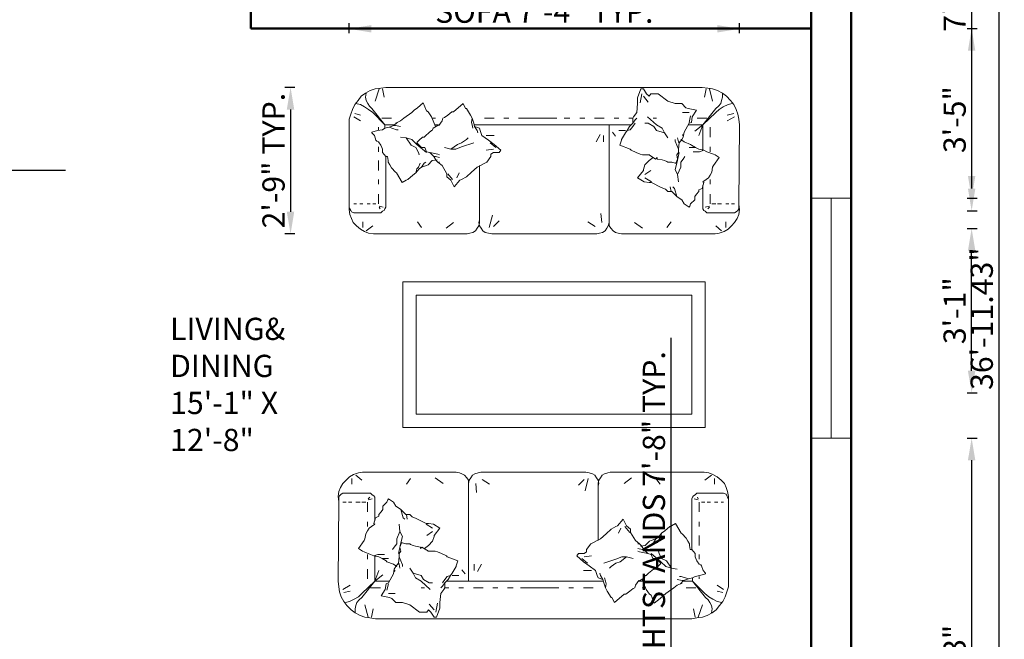
# Model space of a CAD drawing. Units: inches. Extents: x -8 to 396, y -471 to 106.
# Tile 3 of 4: x 167 to 388, y -277 to -138. Entities that reach past the tile are written whole.
import ezdxf

# ---------------------------------------------------------------- set-up
doc = ezdxf.new("R2010")
doc.units = ezdxf.units.IN
for name, color, linetype, lineweight in [('A-ANNO-DIMS', 2, 'Continuous', 18), ('A-AREA-IDEN', 7, 'Continuous', 18), ('A-FLOR-STRS', 7, 'Continuous', 25), ('A-GLAZ', 4, 'Continuous', 18), ('A-WALL', 7, 'Continuous', 50), ('furn', 8, 'Continuous', 18)]:
    doc.layers.add(name, color=color, linetype=linetype, lineweight=lineweight)
doc.styles.get("Standard").update_dxf_attribs({"font": 'arial.ttf'})
doc.dimstyles.new('ISO-25', dxfattribs={"dimtxt": 5, "dimasz": 5, "dimexe": 1.25, "dimexo": 0.625, "dimtad": 1, "dimlunit": 3, "dimtxsty": 'Standard', "dimcen": 2.5, "dimadec": 0, "dimazin": 0, "dimtfac": 1, "dimtmove": 0, "dimatfit": 3, "dimfxl": 1, "dimfxlon": 1, "dimarcsym": 0})

# ---------------------------------------------------------------- blocks, each defined once
blk = doc.blocks.new('sofa-36')
at = {"color": 0, "linetype": 'ByBlock'}
for p, q in [((-0.2, 0.83), (-0.18, 0.85)), ((-0.18, 0.85), (-0.2, 0.83)), ((-0.18, 0.85), (-0.16, 0.87)), ((-0.16, 0.87), (-0.18, 0.85)), ((-0.16, 0.87), (-0.135, 0.885)), ((-0.135, 0.885), (-0.16, 0.87)), ((-0.145, 0.825), (-0.145, 0.86)), ((-0.135, 0.885), (-0.105, 0.895)), ((-0.105, 0.895), (-0.135, 0.885)), ((-0.085, 0.85), (-0.12, 0.88)), ((-0.105, 0.895), (-0.08, 0.9)), ((-0.08, 0.9), (-0.105, 0.895)), ((-0.08, 0.9), (0.495, 0.9)), ((0.495, 0.9), (-0.08, 0.9)), ((0.19, 0.825), (0.215, 0.86)), ((0.415, 0.83), (0.365, 0.865)), ((0.495, 0.9), (0.515, 0.895)), ((0.515, 0.895), (0.495, 0.9)), ((0.515, 0.895), (0.53, 0.89)), ((0.53, 0.89), (0.515, 0.895)), ((0.53, 0.89), (0.545, 0.88)), ((0.545, 0.88), (0.53, 0.89)), ((0.545, 0.88), (0.56, 0.865)), ((0.56, 0.865), (0.545, 0.88)), ((0.56, 0.865), (0.57, 0.85)), ((0.57, 0.85), (0.56, 0.865)), ((0.57, 0.83), (0.575, 0.85)), ((0.57, 0.85), (0.57, 0.83)), ((0.57, 0.83), (0.57, 0.85)), ((0.57, 0.83), (0.575, 0.85)), ((0.575, 0.85), (0.585, 0.865)), ((0.575, 0.85), (0.585, 0.865)), ((0.585, 0.865), (0.595, 0.88)), ((0.585, 0.865), (0.595, 0.88)), ((0.595, 0.88), (0.61, 0.89)), ((0.595, 0.88), (0.61, 0.89)), ((0.61, 0.89), (0.63, 0.895)), ((0.61, 0.89), (0.63, 0.895)), ((0.63, 0.895), (0.645, 0.9)), ((0.63, 0.895), (0.645, 0.9)), ((0.645, 0.9), (0.87, 0.9)), ((0.87, 0.9), (0.645, 0.9)), ((0.655, 0.855), (0.7, 0.825)), ((0.87, 0.9), (1.29, 0.9)), ((1.29, 0.9), (0.87, 0.9)), ((1.28, 0.855), (1.245, 0.82)), ((1.305, 0.86), (1.285, 0.785)), ((1.29, 0.9), (1.31, 0.895)), ((1.31, 0.895), (1.29, 0.9)), ((1.31, 0.895), (1.33, 0.89)), ((1.33, 0.89), (1.31, 0.895)), ((1.33, 0.89), (1.345, 0.88)), ((1.345, 0.88), (1.33, 0.89)), ((1.345, 0.88), (1.355, 0.865)), ((1.355, 0.865), (1.345, 0.88)), ((1.355, 0.865), (1.365, 0.85)), ((1.365, 0.85), (1.355, 0.865)), ((1.365, 0.85), (1.3675, 0.84)), ((1.37, 0.83), (1.365, 0.85)), ((1.365, 0.83), (1.37, 0.85)), ((1.3675, 0.84), (1.37, 0.85)), ((1.37, 0.85), (1.38, 0.865)), ((1.37, 0.85), (1.38, 0.865)), ((1.38, 0.865), (1.39, 0.88)), ((1.38, 0.865), (1.39, 0.88)), ((1.39, 0.88), (1.405, 0.89)), ((1.39, 0.88), (1.405, 0.89)), ((1.405, 0.89), (1.425, 0.895)), ((1.405, 0.89), (1.425, 0.895)), ((1.425, 0.895), (1.44, 0.9)), ((1.425, 0.895), (1.44, 0.9)), ((1.44, 0.9), (2.015, 0.9)), ((2.015, 0.9), (1.44, 0.9)), ((1.525, 0.83), (1.57, 0.865)), ((1.745, 0.825), (1.72, 0.86)), ((2.015, 0.9), (2.045, 0.895)), ((2.045, 0.895), (2.015, 0.9)), ((2.02, 0.85), (2.06, 0.88)), ((2.045, 0.895), (2.07, 0.885)), ((2.07, 0.885), (2.045, 0.895)), ((2.07, 0.885), (2.095, 0.87)), ((2.095, 0.87), (2.07, 0.885)), ((2.08, 0.825), (2.08, 0.86)), ((2.095, 0.87), (2.12, 0.85)), ((2.12, 0.85), (2.095, 0.87)), ((2.12, 0.85), (2.14, 0.83)), ((2.14, 0.83), (2.12, 0.85)), ((-0.225, 0.78), (-0.215, 0.805)), ((-0.215, 0.805), (-0.225, 0.78)), ((-0.215, 0.805), (-0.2, 0.83)), ((-0.2, 0.83), (-0.215, 0.805)), ((0.57, 0.835), (0.57, 0.23)), ((0.57, 0.815), (0.57, 0.83)), ((0.57, 0.815), (0.57, 0.83)), ((0.615, 0.83), (0.62, 0.775)), ((1.365, 0.835), (1.365, 0.48)), ((1.365, 0.815), (1.37, 0.83)), ((1.365, 0.815), (1.365, 0.83)), ((2.14, 0.83), (2.15, 0.805)), ((2.15, 0.805), (2.14, 0.83)), ((2.15, 0.805), (2.16, 0.78)), ((2.16, 0.78), (2.15, 0.805)), ((-0.23, 0.75), (-0.225, 0.78)), ((-0.225, 0.78), (-0.23, 0.75)), ((-0.225, 0.72), (-0.23, 0.75)), ((-0.23, 0.75), (-0.225, 0.72)), ((-0.225, 0.745), (-0.22, 0.755)), ((-0.225, 0.735), (-0.225, 0.745)), ((-0.225, 0.72), (-0.225, 0.735)), ((-0.22, 0.755), (-0.21, 0.765)), ((-0.21, 0.765), (-0.2, 0.77)), ((-0.2, 0.77), (-0.19, 0.77)), ((-0.19, 0.77), (-0.175, 0.77)), ((-0.175, 0.77), (-0.055, 0.77)), ((-0.055, 0.77), (-0.04, 0.77)), ((-0.045, 0.735), (-0.035, 0.745)), ((-0.045, 0.73), (-0.02, 0.735)), ((-0.04, 0.77), (-0.03, 0.77)), ((-0.03, 0.77), (-0.02, 0.76)), ((-0.02, 0.76), (-0.01, 0.755)), ((-0.01, 0.755), (-0.005, 0.745)), ((-0.005, 0.745), (-0.005, 0.735)), ((-0.005, 0.735), (-0.005, 0.72)), ((0.075, 0.73), (0.07, 0.715)), ((0.08, 0.735), (0.075, 0.73)), ((0.11, 0.715), (0.08, 0.735)), ((1.94, 0.735), (1.945, 0.745)), ((1.94, 0.72), (1.94, 0.735)), ((1.945, 0.745), (1.95, 0.755)), ((1.95, 0.755), (1.96, 0.76)), ((1.98, 0.73), (1.955, 0.735)), ((1.96, 0.76), (1.97, 0.77)), ((1.97, 0.77), (1.98, 0.77)), ((1.98, 0.735), (1.975, 0.745)), ((1.98, 0.77), (1.99, 0.77)), ((1.99, 0.77), (2.115, 0.77)), ((2.115, 0.77), (2.125, 0.77)), ((2.125, 0.77), (2.135, 0.77)), ((2.135, 0.77), (2.15, 0.765)), ((2.15, 0.765), (2.155, 0.755)), ((2.155, 0.755), (2.16, 0.745)), ((2.16, 0.78), (2.165, 0.75)), ((2.165, 0.75), (2.16, 0.78)), ((2.16, 0.745), (2.165, 0.735)), ((2.165, 0.75), (2.165, 0.72)), ((2.165, 0.72), (2.165, 0.75)), ((2.165, 0.735), (2.165, 0.72)), ((-0.23, 0.23), (-0.225, 0.72)), ((-0.23, 0.23), (-0.225, 0.72)), ((-0.2, 0.715), (-0.18, 0.715)), ((-0.165, 0.715), (-0.145, 0.715)), ((-0.12, 0.715), (-0.095, 0.715)), ((-0.085, 0.715), (-0.06, 0.715)), ((-0.05, 0.715), (-0.05, 0.655)), ((-0.005, 0.72), (-0.005, 0.6)), ((0.045, 0.67), (0.035, 0.655)), ((0.07, 0.715), (0.045, 0.69)), ((0.045, 0.69), (0.045, 0.68)), ((0.045, 0.68), (0.045, 0.67)), ((0.125, 0.69), (0.11, 0.715)), ((0.14, 0.68), (0.125, 0.69)), ((0.155, 0.67), (0.14, 0.68)), ((0.155, 0.67), (0.17, 0.62)), ((0.185, 0.64), (0.155, 0.67)), ((1.94, 0.42), (1.94, 0.72)), ((1.985, 0.715), (1.985, 0.655)), ((2.02, 0.715), (2, 0.715)), ((2.055, 0.715), (2.035, 0.715)), ((2.1, 0.715), (2.08, 0.715)), ((2.135, 0.715), (2.12, 0.715)), ((2.165, 0.72), (2.165, 0.23)), ((2.165, 0.72), (2.165, 0.23)), ((0, 0.62), (-0.01, 0.585)), ((0.02, 0.63), (0, 0.62)), ((0.035, 0.655), (0.02, 0.64)), ((0.02, 0.64), (0.02, 0.63)), ((0.17, 0.62), (0.18, 0.61)), ((0.185, 0.64), (0.21, 0.64)), ((0.19, 0.64), (0.185, 0.64)), ((0.195, 0.61), (0.19, 0.64)), ((0.21, 0.64), (0.225, 0.625)), ((0.225, 0.625), (0.25, 0.615)), ((0.235, 0.62), (0.235, 0.62)), ((0.25, 0.615), (0.31, 0.585)), ((1.52, 0.61), (1.485, 0.57)), ((1.54, 0.57), (1.52, 0.61)), ((-0.05, 0.595), (-0.05, 0.565)), ((-0.04, 0.555), (-0.05, 0.54)), ((-0.025, 0.565), (-0.04, 0.555)), ((-0.005, 0.58), (-0.025, 0.565)), ((-0.01, 0.585), (-0.005, 0.58)), ((0.15, 0.535), (0.145, 0.58)), ((0.31, 0.585), (0.325, 0.585)), ((0.35, 0.555), (0.31, 0.58)), ((0.325, 0.585), (0.355, 0.58)), ((0.355, 0.58), (0.395, 0.555)), ((0.395, 0.555), (0.36, 0.51)), ((1.445, 0.55), (1.415, 0.52)), ((1.475, 0.565), (1.445, 0.55)), ((1.485, 0.57), (1.475, 0.565)), ((1.505, 0.555), (1.49, 0.525)), ((1.53, 0.565), (1.56, 0.53)), ((1.565, 0.55), (1.54, 0.57)), ((1.565, 0.53), (1.565, 0.55)), ((1.775, 0.54), (1.805, 0.565)), ((1.805, 0.565), (1.815, 0.57)), ((1.815, 0.57), (1.84, 0.585)), ((1.84, 0.585), (1.875, 0.525)), ((1.985, 0.595), (1.985, 0.565)), ((-0.065, 0.49), (-0.07, 0.48)), ((-0.06, 0.52), (-0.065, 0.49)), ((-0.05, 0.54), (-0.06, 0.52)), ((0.15, 0.535), (0.13, 0.49)), ((0.13, 0.49), (0.13, 0.46)), ((0.165, 0.505), (0.15, 0.535)), ((0.155, 0.465), (0.165, 0.505)), ((0.35, 0.535), (0.315, 0.51)), ((0.36, 0.505), (0.35, 0.475)), ((0.36, 0.51), (0.36, 0.505)), ((1.38, 0.49), (1.32, 0.46)), ((1.415, 0.52), (1.38, 0.49)), ((1.595, 0.48), (1.565, 0.53)), ((1.72, 0.49), (1.69, 0.48)), ((1.705, 0.465), (1.72, 0.49)), ((1.72, 0.49), (1.735, 0.5)), ((1.74, 0.49), (1.73, 0.465)), ((1.735, 0.5), (1.755, 0.525)), ((1.75, 0.5), (1.74, 0.49)), ((1.755, 0.525), (1.75, 0.5)), ((1.755, 0.525), (1.775, 0.54)), ((1.875, 0.525), (1.88, 0.52)), ((1.88, 0.52), (1.905, 0.495)), ((1.905, 0.495), (1.915, 0.475)), ((1.985, 0.45), (1.985, 0.51)), ((-0.07, 0.48), (-0.105, 0.43)), ((-0.105, 0.43), (-0.08, 0.415)), ((0.115, 0.44), (0.105, 0.425)), ((0.13, 0.46), (0.115, 0.44)), ((0.14, 0.4), (0.155, 0.465)), ((0.16, 0.465), (0.15, 0.44)), ((0.15, 0.44), (0.155, 0.415)), ((0.165, 0.465), (0.16, 0.465)), ((0.185, 0.46), (0.165, 0.465)), ((0.21, 0.46), (0.185, 0.46)), ((0.215, 0.455), (0.21, 0.46)), ((0.23, 0.45), (0.215, 0.455)), ((0.245, 0.445), (0.23, 0.45)), ((0.275, 0.44), (0.245, 0.445)), ((0.275, 0.43), (0.275, 0.44)), ((0.285, 0.44), (0.275, 0.43)), ((0.325, 0.415), (0.285, 0.44)), ((0.325, 0.45), (0.3, 0.43)), ((0.35, 0.475), (0.325, 0.45)), ((1.32, 0.46), (1.295, 0.425)), ((1.295, 0.425), (1.295, 0.41)), ((1.62, 0.46), (1.595, 0.48)), ((1.615, 0.46), (1.61, 0.46)), ((1.61, 0.43), (1.635, 0.425)), ((1.63, 0.45), (1.62, 0.46)), ((1.655, 0.45), (1.625, 0.445)), ((1.645, 0.425), (1.63, 0.45)), ((1.635, 0.425), (1.645, 0.425)), ((1.645, 0.425), (1.67, 0.4)), ((1.68, 0.475), (1.655, 0.45)), ((1.69, 0.48), (1.68, 0.475)), ((1.695, 0.46), (1.705, 0.465)), ((1.915, 0.475), (1.925, 0.46)), ((1.925, 0.46), (1.925, 0.45)), ((1.925, 0.45), (1.93, 0.425)), ((1.93, 0.425), (1.94, 0.425)), ((1.94, 0.425), (1.96, 0.4)), ((-0.08, 0.415), (-0.07, 0.41)), ((-0.07, 0.41), (-0.03, 0.395)), ((-0.05, 0.365), (-0.05, 0.395)), ((-0.03, 0.395), (-0.01, 0.385)), ((-0.01, 0.385), (0.015, 0.395)), ((-0.01, 0.385), (0.02, 0.38)), ((-0.005, 0.385), (-0.005, 0.23)), ((0.015, 0.395), (0.03, 0.395)), ((0.02, 0.38), (0.04, 0.37)), ((0.03, 0.395), (0.055, 0.395)), ((0.04, 0.37), (0.065, 0.355)), ((0.04, 0.37), (0.065, 0.37)), ((0.065, 0.37), (0.08, 0.37)), ((0.145, 0.38), (0.14, 0.34)), ((0.155, 0.415), (0.145, 0.4)), ((0.145, 0.4), (0.145, 0.38)), ((0.145, 0.38), (0.165, 0.33)), ((0.32, 0.415), (0.325, 0.415)), ((0.355, 0.415), (0.32, 0.415)), ((0.365, 0.415), (0.355, 0.415)), ((0.38, 0.41), (0.365, 0.415)), ((0.405, 0.4), (0.38, 0.41)), ((0.435, 0.385), (0.405, 0.4)), ((0.44, 0.38), (0.435, 0.385)), ((0.505, 0.355), (0.44, 0.38)), ((1.245, 0.4), (1.235, 0.385)), ((1.235, 0.385), (1.275, 0.35)), ((1.28, 0.4), (1.245, 0.4)), ((1.265, 0.37), (1.3, 0.34)), ((1.295, 0.41), (1.28, 0.4)), ((1.28, 0.38), (1.325, 0.385)), ((1.4, 0.34), (1.475, 0.365)), ((1.475, 0.365), (1.51, 0.38)), ((1.54, 0.38), (1.5, 0.35)), ((1.51, 0.38), (1.54, 0.38)), ((1.54, 0.38), (1.58, 0.37)), ((1.62, 0.41), (1.61, 0.415)), ((1.67, 0.4), (1.62, 0.41)), ((1.67, 0.4), (1.69, 0.395)), ((1.69, 0.4), (1.75, 0.35)), ((1.69, 0.395), (1.7, 0.37)), ((1.7, 0.37), (1.72, 0.37)), ((1.72, 0.37), (1.75, 0.34)), ((1.74, 0.4), (1.735, 0.415)), ((1.755, 0.37), (1.74, 0.4)), ((1.785, 0.355), (1.755, 0.37)), ((1.96, 0.4), (1.96, 0.38)), ((1.96, 0.38), (1.965, 0.37)), ((1.965, 0.37), (1.97, 0.355)), ((1.985, 0.365), (1.985, 0.395)), ((-0.05, 0.245), (-0.05, 0.305)), ((0.065, 0.355), (0.07, 0.35)), ((0.07, 0.35), (0.11, 0.335)), ((0.11, 0.335), (0.13, 0.32)), ((0.115, 0.305), (0.11, 0.275)), ((0.125, 0.32), (0.115, 0.305)), ((0.14, 0.34), (0.125, 0.32)), ((0.14, 0.34), (0.145, 0.335)), ((0.145, 0.335), (0.15, 0.31)), ((0.165, 0.33), (0.165, 0.32)), ((0.23, 0.28), (0.21, 0.31)), ((0.47, 0.28), (0.495, 0.32)), ((0.495, 0.325), (0.505, 0.355)), ((0.495, 0.32), (0.495, 0.325)), ((0.605, 0.295), (0.605, 0.335)), ((0.625, 0.29), (0.65, 0.335)), ((1.275, 0.35), (1.31, 0.325)), ((1.31, 0.325), (1.35, 0.295)), ((1.445, 0.32), (1.435, 0.31)), ((1.475, 0.34), (1.445, 0.32)), ((1.5, 0.35), (1.475, 0.34)), ((1.705, 0.305), (1.695, 0.295)), ((1.715, 0.305), (1.705, 0.305)), ((1.735, 0.325), (1.715, 0.305)), ((1.745, 0.335), (1.735, 0.325)), ((1.75, 0.34), (1.745, 0.335)), ((1.75, 0.35), (1.78, 0.32)), ((1.78, 0.32), (1.815, 0.31)), ((1.815, 0.31), (1.785, 0.355)), ((1.815, 0.31), (1.85, 0.305)), ((1.97, 0.355), (1.985, 0.335)), ((1.985, 0.335), (1.995, 0.33)), ((1.995, 0.33), (2, 0.325)), ((2, 0.325), (2.01, 0.295)), ((0.02, 0.295), (-0.005, 0.23)), ((0.045, 0.27), (-0.005, 0.23)), ((0.11, 0.275), (0.08, 0.22)), ((0.12, 0.295), (0.115, 0.29)), ((0.23, 0.28), (0.28, 0.265)), ((0.245, 0.25), (0.23, 0.28)), ((0.28, 0.23), (0.245, 0.25)), ((0.28, 0.265), (0.295, 0.24)), ((0.425, 0.24), (0.44, 0.26)), ((0.44, 0.26), (0.46, 0.265)), ((0.445, 0.24), (0.46, 0.265)), ((0.46, 0.265), (0.47, 0.28)), ((0.51, 0.265), (0.47, 0.265)), ((0.55, 0.275), (0.53, 0.3)), ((1.325, 0.295), (1.275, 0.295)), ((1.35, 0.295), (1.36, 0.265)), ((1.36, 0.265), (1.365, 0.25)), ((1.365, 0.25), (1.395, 0.24)), ((1.38, 0.265), (1.375, 0.28)), ((1.395, 0.24), (1.38, 0.265)), ((1.41, 0.23), (1.405, 0.25)), ((1.65, 0.25), (1.615, 0.23)), ((1.655, 0.265), (1.65, 0.25)), ((1.66, 0.265), (1.655, 0.265)), ((1.675, 0.28), (1.66, 0.265)), ((1.695, 0.295), (1.675, 0.28)), ((1.875, 0.26), (1.865, 0.26)), ((1.92, 0.245), (1.875, 0.26)), ((1.92, 0.245), (1.89, 0.235)), ((1.945, 0.25), (1.92, 0.245)), ((1.96, 0.26), (1.945, 0.25)), ((1.945, 0.25), (1.945, 0.23)), ((1.99, 0.265), (1.96, 0.26)), ((1.985, 0.245), (1.985, 0.26)), ((2.025, 0.275), (1.99, 0.265)), ((2.01, 0.295), (2.025, 0.28)), ((2.025, 0.28), (2.025, 0.275)), ((-0.225, 0.195), (-0.23, 0.23)), ((-0.225, 0.195), (-0.23, 0.23)), ((-0.22, 0.165), (-0.225, 0.195)), ((-0.22, 0.165), (-0.225, 0.195)), ((-0.2, 0.18), (-0.155, 0.205)), ((-0.005, 0.23), (-0.085, 0.13)), ((-0.005, 0.23), (-0.085, 0.155)), ((-0.03, 0.19), (0.03, 0.19)), ((0.085, 0.23), (-0.005, 0.23)), ((0.065, 0.215), (0.06, 0.18)), ((0.08, 0.22), (0.065, 0.215)), ((0.07, 0.175), (0.08, 0.215)), ((0.335, 0.18), (0.28, 0.23)), ((0.28, 0.19), (0.3, 0.19)), ((0.295, 0.24), (0.33, 0.22)), ((0.33, 0.22), (0.35, 0.22)), ((0.41, 0.2), (0.4, 0.19)), ((0.41, 0.22), (0.425, 0.24)), ((0.425, 0.22), (0.41, 0.2)), ((0.42, 0.18), (0.425, 0.19)), ((0.425, 0.22), (0.445, 0.24)), ((0.425, 0.19), (0.425, 0.22)), ((0.45, 0.19), (0.425, 0.19)), ((0.435, 0.23), (0.87, 0.23)), ((0.54, 0.19), (0.51, 0.19)), ((0.6, 0.19), (0.66, 0.19)), ((0.72, 0.19), (0.75, 0.19)), ((0.81, 0.19), (0.845, 0.19)), ((1.395, 0.23), (0.87, 0.23)), ((1.125, 0.19), (0.89, 0.19)), ((1.215, 0.19), (1.185, 0.19)), ((1.335, 0.19), (1.275, 0.19)), ((1.4, 0.22), (1.395, 0.24)), ((1.41, 0.19), (1.4, 0.22)), ((1.415, 0.215), (1.41, 0.23)), ((1.41, 0.19), (1.415, 0.215)), ((1.42, 0.17), (1.41, 0.19)), ((1.58, 0.185), (1.56, 0.17)), ((1.59, 0.19), (1.58, 0.185)), ((1.595, 0.205), (1.59, 0.19)), ((1.615, 0.235), (1.595, 0.205)), ((1.615, 0.23), (1.615, 0.235)), ((1.615, 0.23), (1.615, 0.23)), ((1.64, 0.23), (1.62, 0.23)), ((1.645, 0.215), (1.635, 0.24)), ((1.655, 0.19), (1.635, 0.19)), ((1.66, 0.18), (1.645, 0.215)), ((1.83, 0.19), (1.78, 0.155)), ((1.85, 0.205), (1.83, 0.19)), ((1.845, 0.2), (1.845, 0.2)), ((1.88, 0.235), (1.85, 0.24)), ((1.87, 0.215), (1.85, 0.205)), ((1.89, 0.235), (1.87, 0.215)), ((1.87, 0.215), (1.88, 0.22)), ((1.89, 0.235), (1.88, 0.235)), ((1.885, 0.23), (1.945, 0.23)), ((1.965, 0.19), (1.905, 0.19)), ((1.945, 0.23), (2.025, 0.13)), ((1.945, 0.23), (2.02, 0.155)), ((2.135, 0.18), (2.095, 0.205)), ((2.165, 0.195), (2.155, 0.165)), ((2.165, 0.195), (2.155, 0.165)), ((2.165, 0.23), (2.165, 0.195)), ((2.165, 0.23), (2.165, 0.195)), ((-0.21, 0.135), (-0.22, 0.165)), ((-0.21, 0.135), (-0.22, 0.165)), ((-0.195, 0.105), (-0.21, 0.135)), ((-0.195, 0.105), (-0.21, 0.135)), ((-0.155, 0.17), (-0.195, 0.16)), ((-0.105, 0.135), (-0.13, 0.12)), ((-0.085, 0.155), (-0.105, 0.135)), ((-0.085, 0.13), (-0.1, 0.115)), ((0.06, 0.18), (0.035, 0.14)), ((0.035, 0.14), (0.085, 0.13)), ((0.08, 0.155), (0.12, 0.155)), ((0.085, 0.13), (0.1, 0.125)), ((0.1, 0.125), (0.125, 0.1)), ((0.395, 0.1), (0.4, 0.155)), ((0.4, 0.155), (0.42, 0.18)), ((1.445, 0.13), (1.42, 0.17)), ((1.45, 0.13), (1.445, 0.13)), ((1.465, 0.1), (1.45, 0.13)), ((1.525, 0.15), (1.465, 0.1)), ((1.535, 0.15), (1.525, 0.15)), ((1.56, 0.17), (1.535, 0.15)), ((1.68, 0.15), (1.66, 0.18)), ((1.69, 0.145), (1.68, 0.15)), ((1.71, 0.095), (1.69, 0.145)), ((1.745, 0.125), (1.71, 0.095)), ((1.765, 0.14), (1.745, 0.125)), ((1.78, 0.155), (1.765, 0.14)), ((2.02, 0.155), (2.045, 0.135)), ((2.025, 0.13), (2.04, 0.115)), ((2.045, 0.135), (2.07, 0.12)), ((2.095, 0.17), (2.13, 0.16)), ((2.145, 0.135), (2.13, 0.105)), ((2.145, 0.135), (2.13, 0.105)), ((2.155, 0.165), (2.145, 0.135)), ((2.155, 0.165), (2.145, 0.135)), ((-0.175, 0.08), (-0.195, 0.105)), ((-0.175, 0.08), (-0.195, 0.105)), ((-0.16, 0.105), (-0.185, 0.1)), ((-0.15, 0.055), (-0.175, 0.08)), ((-0.15, 0.055), (-0.175, 0.08)), ((-0.13, 0.12), (-0.16, 0.105)), ((-0.12, 0.08), (-0.125, 0.06)), ((-0.115, 0.1), (-0.12, 0.08)), ((-0.1, 0.115), (-0.115, 0.1)), ((-0.045, 0.01), (-0.065, 0.085)), ((0.125, 0.1), (0.165, 0.1)), ((0.165, 0.1), (0.21, 0.085)), ((0.21, 0.085), (0.27, 0.04)), ((0.36, 0.055), (0.33, 0.09)), ((0.37, 0.04), (0.38, 0.095)), ((0.375, 0.01), (0.395, 0.065)), ((0.395, 0.065), (0.395, 0.1)), ((1.98, 0.01), (2.005, 0.085)), ((2.04, 0.115), (2.05, 0.1)), ((2.05, 0.1), (2.06, 0.08)), ((2.06, 0.08), (2.065, 0.06)), ((2.07, 0.12), (2.095, 0.105)), ((2.11, 0.08), (2.09, 0.055)), ((2.11, 0.08), (2.09, 0.055)), ((2.095, 0.105), (2.125, 0.1)), ((2.13, 0.105), (2.11, 0.08)), ((2.13, 0.105), (2.11, 0.08)), ((-0.125, 0.035), (-0.15, 0.055)), ((-0.125, 0.035), (-0.15, 0.055)), ((-0.125, 0.06), (-0.125, 0.035)), ((-0.095, 0.02), (-0.125, 0.035)), ((-0.095, 0.02), (-0.125, 0.035)), ((-0.065, 0.01), (-0.095, 0.02)), ((-0.065, 0.01), (-0.095, 0.02)), ((-0.035, 0.005), (-0.065, 0.01)), ((-0.035, 0.005), (-0.065, 0.01)), ((0, 0), (-0.035, 0.005)), ((0, 0), (-0.035, 0.005)), ((-0.015, 0.06), (-0.025, 0.01)), ((1.94, 0), (0, 0)), ((1.94, 0), (0, 0)), ((0.27, 0.04), (0.315, 0.04)), ((0.315, 0.04), (0.325, 0.055)), ((0.325, 0.055), (0.34, 0.04)), ((0.34, 0.04), (0.36, 0.01)), ((0.36, 0.01), (0.375, 0.01)), ((1.97, 0.005), (1.94, 0)), ((1.97, 0.005), (1.94, 0)), ((1.95, 0.06), (1.96, 0.01)), ((2.005, 0.01), (1.97, 0.005)), ((2.005, 0.01), (1.97, 0.005)), ((2.035, 0.02), (2.005, 0.01)), ((2.035, 0.02), (2.005, 0.01)), ((2.065, 0.035), (2.035, 0.02)), ((2.065, 0.035), (2.035, 0.02)), ((2.065, 0.06), (2.06, 0.035)), ((2.09, 0.055), (2.065, 0.035)), ((2.09, 0.055), (2.065, 0.035))]:
    blk.add_line(p, q, dxfattribs=at)
blk = doc.blocks.new('*D9')
at = {"layer": 'A-ANNO-DIMS', "color": 0, "lineweight": -2, "transparency": 16777216}
for p, q in [((386.16, 16.55), (388.41, 16.55)), ((387.16, 11.55), (387.16, -421.87)), ((386.16, -426.87), (388.41, -426.87))]:
    blk.add_line(p, q, dxfattribs=at)
at = {"layer": 'A-ANNO-DIMS', "color": 0, "transparency": 16777216}
for points in [[(386.32, 11.55), (387.99, 11.55), (387.16, 16.55)], [(386.32, -421.87), (387.99, -421.87), (387.16, -426.87)]]:
    blk.add_solid(points, dxfattribs=at)
at = {"layer": 'Defpoints', "color": 0, "transparency": 16777216}
for p in [(353.97, 16.55), (353.97, -426.87), (387.16, -426.87)]:
    blk.add_point(p, dxfattribs=at)
at = {"layer": 'A-ANNO-DIMS', "color": 0, "transparency": 16777216, "insert": (383.98, -205.16), "char_height": 5, "attachment_point": 5, "rotation": 90}
blk.add_mtext('36\'-11.43"', dxfattribs=at)
blk = doc.blocks.new('WINDOW-54IN')
blk.add_line((4.5, 54), (4.5, 0))
blk.add_lwpolyline([(0, 54), (9, 54), (9, 0), (0, 0)], close=True)
blk = doc.blocks.new('*D16')
at = {"layer": 'A-ANNO-DIMS', "color": 0, "lineweight": -2, "transparency": 16777216}
for p, q in [((313.46, -318.14), (313.46, -209.45)), ((312.46, -318.14), (314.71, -318.14)), ((313.46, -405.17), (313.46, -323.14)), ((312.46, -410.17), (314.71, -410.17))]:
    blk.add_line(p, q, dxfattribs=at)
at = {"layer": 'A-ANNO-DIMS', "color": 0, "transparency": 16777216}
for points in [[(312.63, -323.14), (314.3, -323.14), (313.46, -318.14)], [(312.63, -405.17), (314.3, -405.17), (313.46, -410.17)]]:
    blk.add_solid(points, dxfattribs=at)
at = {"layer": 'Defpoints', "color": 0, "transparency": 16777216}
for p in [(299.66, -318.14), (313.46, -318.14), (299.66, -410.17)]:
    blk.add_point(p, dxfattribs=at)
at = {"layer": 'A-ANNO-DIMS', "color": 0, "transparency": 16777216, "insert": (310.25, -261.3), "char_height": 5, "attachment_point": 5, "rotation": 90}
blk.add_mtext('BED / NIGHTSTANDS 7\'-8" TYP.', dxfattribs=at)
blk = doc.blocks.new('*D18')
at = {"layer": 'A-ANNO-DIMS', "color": 0, "lineweight": -2, "transparency": 16777216}
for p, q in [((241.05, -140.93), (241.05, -138.68)), ((328.86, -140.93), (328.86, -138.68)), ((323.86, -139.93), (246.05, -139.93))]:
    blk.add_line(p, q, dxfattribs=at)
at = {"layer": 'A-ANNO-DIMS', "color": 0, "transparency": 16777216}
for points in [[(246.05, -139.1), (246.05, -140.76), (241.05, -139.93)], [(323.86, -139.1), (323.86, -140.76), (328.86, -139.93)]]:
    blk.add_solid(points, dxfattribs=at)
at = {"layer": 'Defpoints', "color": 0, "transparency": 16777216}
for p in [(241.05, -139.93), (241.05, -153.1), (328.86, -153.1)]:
    blk.add_point(p, dxfattribs=at)
at = {"layer": 'A-ANNO-DIMS', "color": 0, "transparency": 16777216, "insert": (284.95, -136.72), "char_height": 5, "attachment_point": 5}
blk.add_mtext('SOFA 7\'-4" TYP.', dxfattribs=at)
blk = doc.blocks.new('*D19')
at = {"layer": 'A-ANNO-DIMS', "color": 0, "lineweight": -2, "transparency": 16777216}
for p, q in [((228.88, -153.1), (226.63, -153.1)), ((227.88, -158.1), (227.88, -181.1)), ((228.88, -186.1), (226.63, -186.1))]:
    blk.add_line(p, q, dxfattribs=at)
at = {"layer": 'A-ANNO-DIMS', "color": 0, "transparency": 16777216}
for points in [[(227.04, -158.1), (228.71, -158.1), (227.88, -153.1)], [(227.04, -181.1), (228.71, -181.1), (227.88, -186.1)]]:
    blk.add_solid(points, dxfattribs=at)
at = {"layer": 'Defpoints', "color": 0, "transparency": 16777216}
for p in [(241.05, -153.1), (227.88, -186.1), (241.05, -186.1)]:
    blk.add_point(p, dxfattribs=at)
at = {"layer": 'A-ANNO-DIMS', "color": 0, "transparency": 16777216, "insert": (224.7, -169.6), "char_height": 5, "attachment_point": 5, "rotation": 90}
blk.add_mtext('2\'-9" TYP.', dxfattribs=at)
blk = doc.blocks.new('*D32')
at = {"layer": 'A-ANNO-DIMS', "color": 0, "lineweight": -2, "transparency": 16777216}
for p, q in [((380.06, -88.09), (382.31, -88.09)), ((381.06, -93.09), (381.06, -173.04)), ((380.06, -178.04), (382.31, -178.04))]:
    blk.add_line(p, q, dxfattribs=at)
at = {"layer": 'A-ANNO-DIMS', "color": 0, "transparency": 16777216}
for points in [[(380.22, -93.09), (381.89, -93.09), (381.06, -88.09)], [(380.22, -173.04), (381.89, -173.04), (381.06, -178.04)]]:
    blk.add_solid(points, dxfattribs=at)
at = {"layer": 'Defpoints', "color": 0, "transparency": 16777216}
for p in [(353.97, -88.09), (353.97, -178.04), (381.06, -178.04)]:
    blk.add_point(p, dxfattribs=at)
at = {"layer": 'A-ANNO-DIMS', "color": 0, "transparency": 16777216, "insert": (377.88, -133.06), "char_height": 5, "attachment_point": 5, "rotation": 90}
blk.add_mtext('7\'-6"', dxfattribs=at)
blk = doc.blocks.new('*D33')
at = {"layer": 'A-ANNO-DIMS', "color": 0, "lineweight": -2, "transparency": 16777216}
for p, q in [((380.06, -232.04), (382.31, -232.04)), ((381.06, -237.04), (381.06, -326.13)), ((380.06, -331.13), (382.31, -331.13))]:
    blk.add_line(p, q, dxfattribs=at)
at = {"layer": 'A-ANNO-DIMS', "color": 0, "transparency": 16777216}
for points in [[(380.22, -237.04), (381.89, -237.04), (381.06, -232.04)], [(380.22, -326.13), (381.89, -326.13), (381.06, -331.13)]]:
    blk.add_solid(points, dxfattribs=at)
at = {"layer": 'Defpoints', "color": 0, "transparency": 16777216}
for p in [(353.97, -232.04), (353.97, -331.13), (381.06, -331.13)]:
    blk.add_point(p, dxfattribs=at)
at = {"layer": 'A-ANNO-DIMS', "color": 0, "transparency": 16777216, "insert": (377.88, -281.58), "char_height": 5, "attachment_point": 5, "rotation": 90}
blk.add_mtext('8\'-3"', dxfattribs=at)
blk = doc.blocks.new('*D37')
at = {"layer": 'A-ANNO-DIMS', "color": 0, "lineweight": -2, "transparency": 16777216}
for p, q in [((380.06, -184.87), (382.31, -184.87)), ((381.06, -216.87), (381.06, -189.87)), ((380.06, -221.87), (382.31, -221.87))]:
    blk.add_line(p, q, dxfattribs=at)
at = {"layer": 'A-ANNO-DIMS', "color": 0, "transparency": 16777216}
for points in [[(380.22, -189.87), (381.89, -189.87), (381.06, -184.87)], [(380.22, -216.87), (381.89, -216.87), (381.06, -221.87)]]:
    blk.add_solid(points, dxfattribs=at)
at = {"layer": 'Defpoints', "color": 0, "transparency": 16777216}
for p in [(158.97, -184.87), (381.06, -184.87), (158.97, -221.87)]:
    blk.add_point(p, dxfattribs=at)
at = {"layer": 'A-ANNO-DIMS', "color": 0, "transparency": 16777216, "insert": (377.88, -203.37), "char_height": 5, "attachment_point": 5, "rotation": 90}
blk.add_mtext('3\'-1"', dxfattribs=at)
blk = doc.blocks.new('*D38')
at = {"layer": 'A-ANNO-DIMS', "color": 0, "lineweight": -2, "transparency": 16777216}
for p, q in [((380.06, -139.87), (382.31, -139.87)), ((381.06, -144.87), (381.06, -175.87)), ((380.06, -180.87), (382.31, -180.87))]:
    blk.add_line(p, q, dxfattribs=at)
at = {"layer": 'A-ANNO-DIMS', "color": 0, "transparency": 16777216}
for points in [[(380.22, -144.87), (381.89, -144.87), (381.06, -139.87)], [(380.22, -175.87), (381.89, -175.87), (381.06, -180.87)]]:
    blk.add_solid(points, dxfattribs=at)
at = {"layer": 'Defpoints', "color": 0, "transparency": 16777216}
for p in [(158.97, -139.87), (158.97, -180.87), (381.06, -180.87)]:
    blk.add_point(p, dxfattribs=at)
at = {"layer": 'A-ANNO-DIMS', "color": 0, "transparency": 16777216, "insert": (377.88, -160.37), "char_height": 5, "attachment_point": 5, "rotation": 90}
blk.add_mtext('3\'-5"', dxfattribs=at)
blk = doc.blocks.new('*D46')
at = {"layer": 'A-ANNO-DIMS', "color": 0, "lineweight": -2, "transparency": 16777216}
for p, q in [((185.28, -452.96), (185.28, -455.21)), ((215.28, -452.96), (215.28, -455.21)), ((190.28, -453.96), (210.28, -453.96))]:
    blk.add_line(p, q, dxfattribs=at)
at = {"layer": 'A-ANNO-DIMS', "color": 0, "transparency": 16777216}
for points in [[(190.28, -453.13), (190.28, -454.8), (185.28, -453.96)], [(210.28, -453.13), (210.28, -454.8), (215.28, -453.96)]]:
    blk.add_solid(points, dxfattribs=at)
at = {"layer": 'Defpoints', "color": 0, "transparency": 16777216}
for p in [(185.28, -87.87), (215.28, -87.87), (215.28, -453.96)]:
    blk.add_point(p, dxfattribs=at)
at = {"layer": 'A-ANNO-DIMS', "color": 0, "transparency": 16777216, "insert": (200.28, -450.79), "char_height": 5, "attachment_point": 5}
blk.add_mtext('2\'-6"', dxfattribs=at)
blk = doc.blocks.new('*D48')
at = {"layer": 'A-ANNO-DIMS', "color": 0, "lineweight": -2, "transparency": 16777216}
for p, q in [((169.97, -452.96), (169.97, -455.21)), ((190.97, -452.96), (190.97, -455.21)), ((174.97, -453.96), (185.97, -453.96))]:
    blk.add_line(p, q, dxfattribs=at)
at = {"layer": 'A-ANNO-DIMS', "color": 0, "transparency": 16777216}
for points in [[(174.97, -453.13), (174.97, -454.8), (169.97, -453.96)], [(185.97, -453.13), (185.97, -454.8), (190.97, -453.96)]]:
    blk.add_solid(points, dxfattribs=at)
at = {"layer": 'Defpoints', "color": 0, "transparency": 16777216}
for p in [(169.97, 0.13), (190.97, 0.13), (190.97, -453.96)]:
    blk.add_point(p, dxfattribs=at)
at = {"layer": 'A-ANNO-DIMS', "color": 0, "transparency": 16777216, "insert": (180.47, -450.79), "char_height": 5, "attachment_point": 5}
blk.add_mtext('1\'-9"', dxfattribs=at)
blk = doc.blocks.new('*D50')
at = {"layer": 'A-ANNO-DIMS', "color": 0, "lineweight": -2, "transparency": 16777216}
for p, q in [((166.97, 94.22), (166.97, 96.47)), ((202.97, 94.22), (202.97, 96.47)), ((171.97, 95.22), (197.97, 95.22))]:
    blk.add_line(p, q, dxfattribs=at)
at = {"layer": 'A-ANNO-DIMS', "color": 0, "transparency": 16777216}
for points in [[(171.97, 96.05), (171.97, 94.38), (166.97, 95.22)], [(197.97, 96.05), (197.97, 94.38), (202.97, 95.22)]]:
    blk.add_solid(points, dxfattribs=at)
at = {"layer": 'Defpoints', "color": 0, "transparency": 16777216}
for p in [(202.97, 95.22), (166.97, -317.87), (202.97, -317.87)]:
    blk.add_point(p, dxfattribs=at)
at = {"layer": 'A-ANNO-DIMS', "color": 0, "transparency": 16777216, "insert": (184.97, 98.4), "char_height": 5, "attachment_point": 5}
blk.add_mtext('3\'-0"', dxfattribs=at)
blk = doc.blocks.new('*D52')
at = {"layer": 'A-ANNO-DIMS', "color": 0, "lineweight": -2, "transparency": 16777216}
for p, q in [((304.97, 94.22), (304.97, 96.47)), ((340.97, 94.22), (340.97, 96.47)), ((309.97, 95.22), (335.97, 95.22))]:
    blk.add_line(p, q, dxfattribs=at)
at = {"layer": 'A-ANNO-DIMS', "color": 0, "transparency": 16777216}
for points in [[(309.97, 96.05), (309.97, 94.38), (304.97, 95.22)], [(335.97, 96.05), (335.97, 94.38), (340.97, 95.22)]]:
    blk.add_solid(points, dxfattribs=at)
at = {"layer": 'Defpoints', "color": 0, "transparency": 16777216}
for p in [(340.97, 95.22), (304.97, -293.87), (340.97, -293.87)]:
    blk.add_point(p, dxfattribs=at)
at = {"layer": 'A-ANNO-DIMS', "color": 0, "transparency": 16777216, "insert": (322.97, 98.4), "char_height": 5, "attachment_point": 5}
blk.add_mtext('3\'-0"', dxfattribs=at)

msp = doc.modelspace()

# ---------------------------------------------------------------- linework, layer by layer
at = {"layer": 'A-FLOR-STRS'}
msp.add_line((177.259, -171.819), (63.931, -171.819), dxfattribs=at)
at = {"layer": 'A-WALL'}
for p, q in [((353.966, 17.126), (353.966, -426.874)), ((218.966, -139.874), (218.966, 8.126)), ((344.966, 8.126), (344.966, -417.874)), ((218.966, -139.874), (344.966, -139.874))]:
    msp.add_line(p, q, dxfattribs=at)
at = {"layer": 'furn'}
for points in [[(253.12, -196.903), (321.141, -196.903), (321.141, -229.672), (253.12, -229.672)], [(256.12, -199.903), (318.141, -199.903), (318.141, -226.672), (256.12, -226.672)]]:
    msp.add_lwpolyline(points, close=True, dxfattribs=at)

# ---------------------------------------------------------------- block references
at = {"layer": 'A-GLAZ'}
msp.add_blockref('WINDOW-54IN', (344.966, -232.037), dxfattribs=at)
at = {"layer": 'furn', "xscale": 36.66436083614781, "yscale": 36.66436083614781, "zscale": 36.66436083614781, "rotation": 180}
msp.add_blockref('sofa-36', (320.427, -153.102), dxfattribs=at)
at = {"layer": 'furn', "xscale": 36.66436083614781, "yscale": 36.66436083614781, "zscale": 36.66436083614781}
msp.add_blockref('sofa-36', (246.992, -272.683), dxfattribs=at)

# ---------------------------------------------------------------- texts
at = {"layer": 'A-AREA-IDEN', "insert": (200.789, -204.956), "char_height": 5, "attachment_point": 1}
msp.add_mtext_dynamic_manual_height_columns('LIVING& DINING\\P15\'-1" X 12\'-8"', width=43.27019, gutter_width=12.5, heights=[0], dxfattribs=at)

# ---------------------------------------------------------------- dimensions: what is measured, and where the dimension line sits
at = {"layer": 'A-ANNO-DIMS'}
for base, p1, p2, picture, middle in [((202.966, 95.216), (166.966, -317.874), (202.966, -317.874), '*D50', (184.966, 98.396)), ((340.966, 95.216), (304.966, -293.874), (340.966, -293.874), '*D52', (322.966, 98.396)), ((190.966, -453.964), (169.966, 0.126), (190.966, 0.126), '*D48', (180.466, -450.786)), ((215.282, -453.964), (185.282, -87.874), (215.282, -87.874), '*D46', (200.282, -450.786))]:
    dim = msp.add_linear_dim(base=base, p1=p1, p2=p2, dimstyle='ISO-25', override={"dimdec": 1, "dimlfac": 1, "dimrnd": 0, "dimzin": 1, "dimdsep": 46, "dimlunit": 4, "dimfrac": 2}, dxfattribs=at)
    dim.commit()
    dim.dimension.update_dxf_attribs({"geometry": picture, "text_midpoint": middle})
for base, p1, p2, override, picture, middle in [((387.1551, -426.874), (353.9656, 16.5511), (353.9656, -426.874), {"dimclrd": 0, "dimclre": 0, "dimclrt": 0}, '*D9', (383.9755, -205.1614)), ((381.056, -178.037), (353.966, -88.09), (353.966, -178.037), {"dimdec": 1, "dimlfac": 1, "dimrnd": 0, "dimzin": 1, "dimdsep": 46, "dimlunit": 4, "dimfrac": 2}, '*D32', (377.878, -133.064)), ((381.056, -180.874), (158.966, -139.874), (158.966, -180.874), {"dimdec": 1, "dimlfac": 1, "dimrnd": 0, "dimzin": 1, "dimdsep": 46, "dimlunit": 4, "dimfrac": 2}, '*D38', (377.876, -160.374)), ((381.056, -184.874), (158.966, -221.874), (158.966, -184.874), {"dimdec": 1, "dimlfac": 1, "dimrnd": 0, "dimzin": 1, "dimdsep": 46, "dimlunit": 4, "dimfrac": 2}, '*D37', (377.876, -203.374)), ((381.056, -331.125), (353.966, -232.037), (353.966, -331.125), {"dimdec": 1, "dimlfac": 1, "dimrnd": 0, "dimzin": 1, "dimdsep": 46, "dimlunit": 4, "dimfrac": 2}, '*D33', (377.876, -281.581))]:
    dim = msp.add_linear_dim(base=base, p1=p1, p2=p2, angle=90, dimstyle='ISO-25', override=override, dxfattribs=at)
    dim.commit()
    dim.dimension.update_dxf_attribs({"geometry": picture, "text_midpoint": middle})
for base, p1, p2, angle, text, picture, middle in [((241.049, -139.93), (328.86, -153.102), (241.049, -153.102), 180, 'SOFA <> TYP.', '*D18', (284.954, -136.718)), ((227.877, -186.1), (241.049, -153.102), (241.049, -186.1), 270, '<> TYP.', '*D19', (224.699, -169.601)), ((313.462, -318.141), (299.658, -410.169), (299.658, -318.141), 90, 'BED / NIGHTSTANDS <> TYP.', '*D16', (310.252, -261.295))]:
    dim = msp.add_linear_dim(base=base, p1=p1, p2=p2, angle=angle, text=text, dimstyle='ISO-25', override={"dimdec": 1, "dimlfac": 1, "dimrnd": 0, "dimzin": 1, "dimdsep": 46, "dimlunit": 4, "dimfrac": 2}, dxfattribs=at)
    dim.commit()
    dim.dimension.update_dxf_attribs({"geometry": picture, "text_midpoint": middle})

doc.saveas('drawing.dxf')
